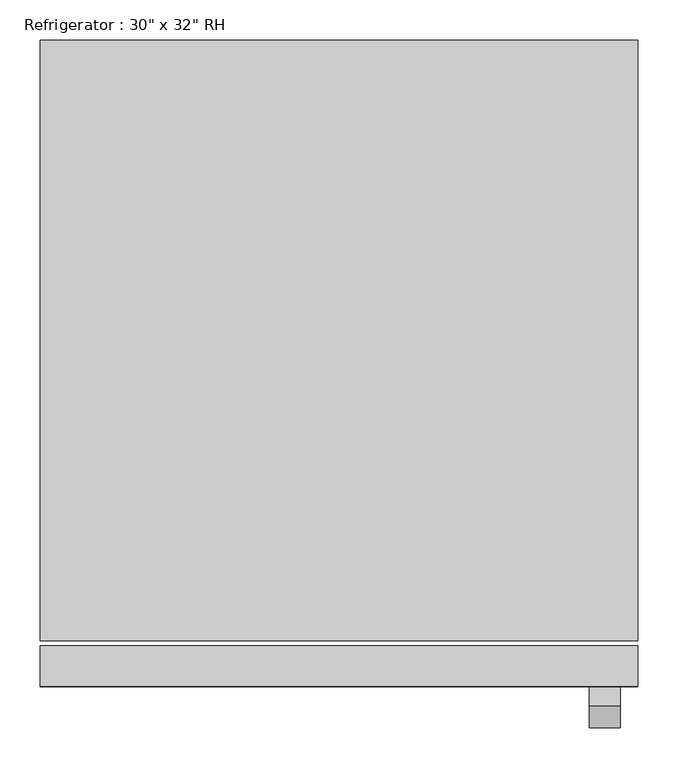
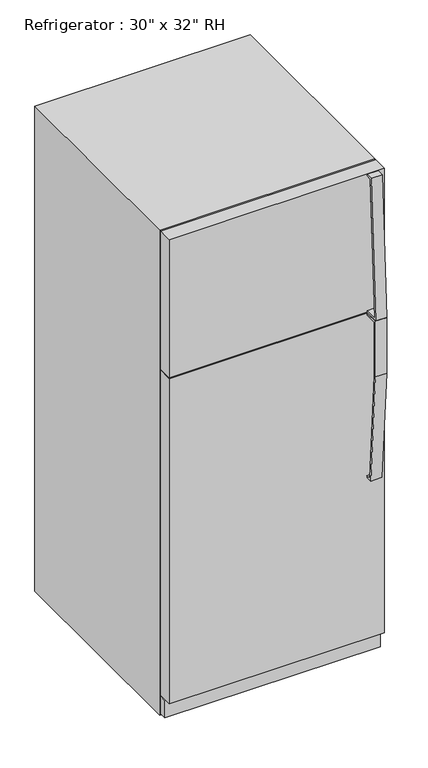
"""IFC4 building model written with IfcOpenShell, lengths in millimetres: proxy geometry."""

from ifc_helpers import new_model, si_unit, frame, origin, origin_with_axes, place, context, project, spatial, polyline, outline, extrude, source, transform, mapped, element, save


def proxy_a13a33b2(model_context):
    return source(origin(), model_context, "Body", "SweptSolid", [
        extrude(outline(polyline([(-417.9010285, 1262.0625), (-462.3510285, 1262.0625), (-462.3510285, 1065.4342469), (-434.8723987, 672.4715334), (-417.9010285, 672.4715334), (-417.9010285, 666.1370017), (-440.7949512, 666.1370017), (-468.7010285, 1065.2125), (-468.7010285, 1268.4125), (-417.9010285, 1268.4125), (-417.9010285, 1262.0625)])), frame((312.7375, 0.0, 0.0), z_axis=(1.0, 0.0, 0.0), x_axis=(0.0, 1.0, 0.0)), (0.0, 0.0, 1.0), 38.4332978),
        extrude(outline(polyline([(-442.739413, 1778.0), (-418.6780855, 1778.0), (-418.6780855, 1771.65), (-437.5263449, 1771.65), (-463.4007207, 1277.9375), (-418.6780855, 1277.9375), (-418.6780855, 1271.5875), (-469.2793675, 1271.5875), (-442.739413, 1778.0)])), frame((312.7375, 0.0, 0.0), z_axis=(1.0, 0.0, 0.0), x_axis=(0.0, 1.0, 0.0)), (0.0, 0.0, 1.0), 38.4332978),
        extrude(outline(polyline([(373.0625, -367.1010285), (373.0625, -392.5010285), (-373.0625, -392.5010285), (-373.0625, -367.1010285), (373.0625, -367.1010285)])), frame((0.0, 0.0, 9.3816357), z_axis=(0.0, 0.0, 1.0), x_axis=(1.0, 0.0, 0.0)), (0.0, 0.0, 1.0), 63.5),
        extrude(outline(polyline([(373.0625, -367.1010285), (373.0625, -417.9010285), (-373.0625, -417.9010285), (-373.0625, -367.1010285), (373.0625, -367.1010285)])), frame((0.0, 0.0, 76.2), z_axis=(0.0, 0.0, 1.0), x_axis=(1.0, 0.0, 0.0)), (0.0, 0.0, 1.0), 1192.2125),
        extrude(outline(polyline([(373.0625, -367.1010285), (373.0625, -417.9010285), (-373.0625, -417.9010285), (-373.0625, -367.1010285), (373.0625, -367.1010285)])), frame((0.0, 0.0, 1271.5875), z_axis=(0.0, 0.0, 1.0), x_axis=(1.0, 0.0, 0.0)), (0.0, 0.0, 1.0), 506.4125),
        extrude(outline(polyline([(373.0625, 388.5489715), (373.0625, -360.7510285), (-373.0625, -360.7510285), (-373.0625, 388.5489715), (373.0625, 388.5489715)])), origin_with_axes(), (0.0, 0.0, 1.0), 1778.0),
    ])


if __name__ == "__main__":
    model = new_model("IFC4")
    model_context = context("Model", 3, world=origin())
    ifc_project = project(units=[si_unit("LENGTHUNIT", "METRE", prefix="MILLI")], contexts=[model_context])
    site = spatial("IfcSite", under=ifc_project)
    building = spatial("IfcBuilding", under=site)
    placement = place(None, origin())
    proxy_shape = proxy_a13a33b2(model_context)
    element("IfcBuildingElementProxy", 1, Name="Refrigerator : 30\" x 32\" RH", ObjectType="Refrigerator : 30\" x 32\" RH", at=placement, inside=building, context=model_context, shape_type="MappedRepresentation", body=[
        mapped(proxy_shape, transform((0.0, 0.0, 0.0), x_axis=(1.0, 0.0, 0.0), y_axis=(0.0, 1.0, 0.0), z_axis=(0.0, 0.0, 1.0))),
    ])
    save(model, "model.ifc")

# Revit data of these elements
# Type "Refrigerator : 30\" x 32\" RH"
#   Label = "REF."
#   Assembly Code = "E1090400"
#   Depth = 2' - 7 3/4"
#   Handle = 2' - 3"
#   Height = 5' - 10"
#   Rear Clearance = 0' - 2"
#   Top Door Height = 1' - 8"
#   Width = 2' - 5 3/8"
#   Material = Copper
#   Default Elevation = 0
# Element 1 (IfcBuildingElementProxy, "Refrigerator : 30\" x 32\" RH")
#   Materials on its faces: "Copper", "Steel, Chrome Plated"
# Materials
#   "Copper": class "Metal", colour RGB 0 0 0, transparency 0, Description = "Copper, matte finish", Cost = 0
#   "Steel, Chrome Plated": class "Metal", colour RGB 17 17 17, transparency 0, Description = "Chromiuim plated steel", Cost = 0
